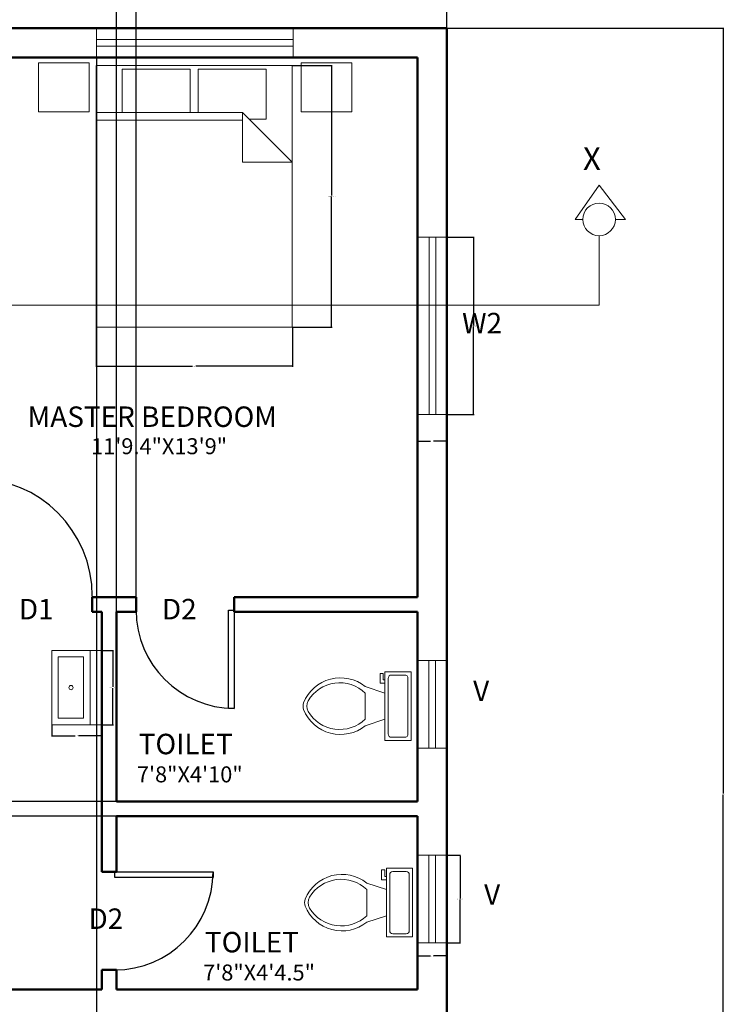
# Model space of a CAD drawing. Units: inches. Extents: x 7359 to 7979, y 33027 to 34263.
# Tile 18 of 32: x 7764 to 7979, y 33329 to 33630. Entities that reach past the tile are written whole.
import ezdxf

# ---------------------------------------------------------------- set-up
doc = ezdxf.new("R2010")
doc.units = ezdxf.units.IN
for name, color, linetype, lineweight in [('A-ANNO-DIMS', 2, 'Continuous', 18), ('A-ANNO-SYMB', 7, 'Continuous', 18), ('A-ANNO-TEXT', 3, 'Continuous', 18), ('A-AREA-IDEN', 7, 'Continuous', 18), ('A-DOOR', 3, 'Continuous', 25), ('A-FLOR-FIXT', 9, 'Continuous', 18), ('A-FURN', 8, 'Continuous', 18), ('A-GLAZ', 4, 'Continuous', 18), ('A-WALL', 7, 'Continuous', 50)]:
    doc.layers.add(name, color=color, linetype=linetype, lineweight=lineweight)
doc.styles.get("Standard").update_dxf_attribs({"font": 'arial.ttf'})
doc.dimstyles.get("Standard").update_dxf_attribs({"dimtxt": 0.18, "dimasz": 0.18, "dimexe": 0.18, "dimexo": 0.0625, "dimgap": 0.09, "dimtad": 0, "dimtih": 1, "dimtoh": 1, "dimdec": 4, "dimzin": 0, "dimdsep": 46, "dimtxsty": 'Standard', "dimcen": 0.09, "dimadec": 0, "dimazin": 0, "dimtfac": 1, "dimtdec": 4, "dimtofl": 0, "dimtmove": 0, "dimatfit": 3, "dimfxl": 1, "dimtolj": 1, "dimtzin": 0, "dimarcsym": 0})

# ---------------------------------------------------------------- blocks, each defined once
blk = doc.blocks.new('*U2')
for p, q in [((0, 0), (0, -100)), ((750, 0), (750, -100))]:
    blk.add_line(p, q)
blk.add_lwpolyline([(0, 0), (0, 750), (43.75, 750), (43.75, 0)], close=True)
blk.add_arc((0, 0), 750, 0, 90)
blk = doc.blocks.new('Bed - Queen')
for p, q in [((0, -80.00003), (0, 0)), ((0, 0), (59.99999, 0)), ((59.99999, 0), (59.99999, -80.00003)), ((7.99999, -1.2), (28.79998, -1.2)), ((7.99999, -14.4), (7.99999, -1.2)), ((28.79998, -1.2), (28.79998, -14.4)), ((31.19999, -1.2), (51.99999, -1.2)), ((31.19999, -14.4), (31.19999, -1.2)), ((51.99999, -1.2), (51.99999, -16.4)), ((0, -14.4), (44.8, -14.4)), ((59.99999, -29.6), (44.8, -14.4)), ((44.8, -14.4), (44.8, -29.6)), ((44.8, -16.8), (0, -16.8)), ((51.99999, -16.4), (46.79936, -16.4)), ((44.8, -29.6), (59.99999, -29.6)), ((59.99999, -80.00003), (0, -80.00003))]:
    blk.add_line(p, q)
blk = doc.blocks.new('Toilet - top')
for p, q in [((9.5, -6), (9.5, -2)), ((-10, -8.5), (-8, -8.5)), ((-10, -9.5), (-10, -8.5)), ((-8, -8.5), (-8, -8)), ((-7, -8), (-7, -9.5)), ((-4, -8), (-6, -14)), ((4, -8), (6, -14)), ((-7, -9.5), (-10, -9.5)), ((4, -14), (-4, -14))]:
    blk.add_line(p, q)
blk.add_lwpolyline([(10.5, -8), (10.5, 0), (-10.5, 0), (-10.5, -8)], close=True)
for points in [[(-9.5, -2), (-9.5, -6)], [(8.5, -1), (-8.5, -1)], [(-8.5, -7), (8.5, -7)]]:
    blk.add_lwpolyline(points)
for centre, radius, start, end in [((-8.62, -1.88), 0.884, 81.8699, 188.1301), ((8.62, -1.88), 0.884, 351.8699, 98.1301), ((-8.62, -6.12), 0.884, 171.8699, 278.1301), ((8.62, -6.12), 0.884, 261.8699, 8.1301), ((3.52, -21.58), 12.17, 141.4691, 247.9714), ((4.2, -21.82), 11.33, 136.3677, 238.9468), ((-3.52, -21.58), 12.17, 292.0284, 38.5307), ((-4.2, -21.82), 11.33, 301.053, 43.6321), ((0, -27.88), 4, 245.7318, 294.2682), ((0, -29), 4, 254.8605, 285.1395)]:
    blk.add_arc(centre, radius, start, end)
blk = doc.blocks.new('TABLE-BEDSIDE')
blk.add_lwpolyline([(0, 15), (15.54, 15), (15.54, 0), (0, 0)], close=True)
blk = doc.blocks.new('BASIN-WALL')
for points in [[(11.75, 22.71), (0, 22.71), (0, 0), (11.75, 0)], [(15.29, 22.71), (11.75, 22.71), (11.75, 0), (15.29, 0)], [(9.75, 20.71), (2, 20.71), (2, 2), (9.75, 2)]]:
    blk.add_lwpolyline(points, close=True)
blk.add_circle((5.88, 11.36), 0.663)
blk = doc.blocks.new('SECTION-HEAD')
for p, q in [((0, 4.98), (7.32, 15.43)), ((7.32, 15.43), (15.39, 4.98)), ((2.34, 4.98), (0, 4.98)), ((12.3, 4.98), (15.39, 4.98))]:
    blk.add_line(p, q)
blk.add_circle((7.32, 4.98), 4.98)
blk = doc.blocks.new('WINDOW-W2-BEDROOM')
for p, q in [((0, 0), (0, 9)), ((60.05, 0), (60.05, 9)), ((60.05, 5.5), (0, 5.5)), ((60.05, 3.5), (0, 3.5))]:
    blk.add_line(p, q)
blk = doc.blocks.new('WINDOW-W2-SIDE')
for p, q in [((0, 54.21), (9, 54.21)), ((3.61, 0), (3.61, 54.21)), ((5.61, 0), (5.61, 54.21)), ((0.22, 0), (9, 0))]:
    blk.add_line(p, q)
blk = doc.blocks.new('VENT-V')
for p, q in [((0, 26.78), (9, 26.78)), ((3.5, 0), (3.5, 26.78)), ((5.5, 0), (5.5, 26.78)), ((0, 0), (9, 0))]:
    blk.add_line(p, q)
blk = doc.blocks.new('*D28')
at = {"layer": 'A-ANNO-DIMS', "color": 0, "lineweight": -2, "transparency": 16777216}
for p, q in [((7846.94, 33615.76), (7859.06, 33615.76)), ((7858.88, 33615.58), (7858.88, 33575.95)), ((7858.88, 33535.94), (7858.88, 33575.57)), ((7846.94, 33535.76), (7859.06, 33535.76))]:
    blk.add_line(p, q, dxfattribs=at)
at = {"layer": 'A-ANNO-DIMS', "color": 0, "transparency": 16777216}
for points in [[(7858.85, 33615.58), (7858.91, 33615.58), (7858.88, 33615.76)], [(7858.85, 33535.94), (7858.91, 33535.94), (7858.88, 33535.76)]]:
    blk.add_solid(points, dxfattribs=at)
at = {"layer": 'Defpoints', "color": 0, "transparency": 16777216}
for p in [(7846.88, 33615.76), (7858.88, 33615.76), (7846.88, 33535.76)]:
    blk.add_point(p, dxfattribs=at)
at = {"layer": 'A-ANNO-DIMS', "color": 0, "transparency": 16777216, "insert": (7858.88, 33575.76), "char_height": 0.18, "attachment_point": 5}
blk.add_mtext('\\A1;QUEEN BED 80 TYP.', dxfattribs=at)
blk = doc.blocks.new('*D29')
at = {"layer": 'A-ANNO-DIMS', "color": 0, "lineweight": -2, "transparency": 16777216}
for p, q in [((7786.88, 33535.7), (7786.88, 33523.58)), ((7846.88, 33535.7), (7846.88, 33523.58)), ((7787.06, 33523.76), (7816.35, 33523.76)), ((7846.7, 33523.76), (7817.4, 33523.76))]:
    blk.add_line(p, q, dxfattribs=at)
at = {"layer": 'A-ANNO-DIMS', "color": 0, "transparency": 16777216}
for points in [[(7787.06, 33523.79), (7787.06, 33523.73), (7786.88, 33523.76)], [(7846.7, 33523.79), (7846.7, 33523.73), (7846.88, 33523.76)]]:
    blk.add_solid(points, dxfattribs=at)
at = {"layer": 'Defpoints', "color": 0, "transparency": 16777216}
for p in [(7786.88, 33535.76), (7846.88, 33535.76), (7846.88, 33523.76)]:
    blk.add_point(p, dxfattribs=at)
at = {"layer": 'A-ANNO-DIMS', "color": 0, "transparency": 16777216, "insert": (7816.88, 33523.76), "char_height": 0.18, "attachment_point": 5}
blk.add_mtext('\\A1;60 TYP.', dxfattribs=at)
blk = doc.blocks.new('*D34')
at = {"layer": 'A-ANNO-DIMS', "color": 0, "lineweight": -2, "transparency": 16777216}
for p, q in [((7894.19, 33374.26), (7898.32, 33374.26)), ((7898.14, 33374.08), (7898.14, 33361.05)), ((7898.14, 33347.66), (7898.14, 33360.69)), ((7894.19, 33347.48), (7898.32, 33347.48))]:
    blk.add_line(p, q, dxfattribs=at)
at = {"layer": 'A-ANNO-DIMS', "color": 0, "transparency": 16777216}
for points in [[(7898.11, 33374.08), (7898.17, 33374.08), (7898.14, 33374.26)], [(7898.11, 33347.66), (7898.17, 33347.66), (7898.14, 33347.48)]]:
    blk.add_solid(points, dxfattribs=at)
at = {"layer": 'Defpoints', "color": 0, "transparency": 16777216}
for p in [(7894.13, 33374.26), (7898.14, 33374.26), (7894.13, 33347.48)]:
    blk.add_point(p, dxfattribs=at)
at = {"layer": 'A-ANNO-DIMS', "color": 0, "transparency": 16777216, "insert": (7898.14, 33360.87), "char_height": 0.18, "attachment_point": 5}
blk.add_mtext('\\A1;VENT V 27 TYP.', dxfattribs=at)
blk = doc.blocks.new('*D35')
at = {"layer": 'A-ANNO-DIMS', "color": 0, "lineweight": -2, "transparency": 16777216}
for p, q in [((7885.13, 33347.42), (7885.13, 33343.28)), ((7894.13, 33347.42), (7894.13, 33343.28)), ((7885.31, 33343.46), (7889.17, 33343.46)), ((7893.95, 33343.46), (7890.08, 33343.46))]:
    blk.add_line(p, q, dxfattribs=at)
at = {"layer": 'A-ANNO-DIMS', "color": 0, "transparency": 16777216}
for points in [[(7885.31, 33343.49), (7885.31, 33343.43), (7885.13, 33343.46)], [(7893.95, 33343.49), (7893.95, 33343.43), (7894.13, 33343.46)]]:
    blk.add_solid(points, dxfattribs=at)
at = {"layer": 'Defpoints', "color": 0, "transparency": 16777216}
for p in [(7885.13, 33347.48), (7894.13, 33347.48), (7894.13, 33343.46)]:
    blk.add_point(p, dxfattribs=at)
at = {"layer": 'A-ANNO-DIMS', "color": 0, "transparency": 16777216, "insert": (7889.63, 33343.46), "char_height": 0.18, "attachment_point": 5}
blk.add_mtext('\\A1;9 TYP.', dxfattribs=at)
blk = doc.blocks.new('*D48')
at = {"layer": 'A-ANNO-DIMS', "color": 0, "lineweight": -2, "transparency": 16777216}
for p, q in [((7788.69, 33436.88), (7792.21, 33436.88)), ((7792.03, 33436.7), (7792.03, 33425.7)), ((7792.03, 33414.34), (7792.03, 33425.34)), ((7788.69, 33414.16), (7792.21, 33414.16))]:
    blk.add_line(p, q, dxfattribs=at)
at = {"layer": 'A-ANNO-DIMS', "color": 0, "transparency": 16777216}
for points in [[(7792, 33436.7), (7792.06, 33436.7), (7792.03, 33436.88)], [(7792, 33414.34), (7792.06, 33414.34), (7792.03, 33414.16)]]:
    blk.add_solid(points, dxfattribs=at)
at = {"layer": 'Defpoints', "color": 0, "transparency": 16777216}
for p in [(7788.63, 33436.88), (7792.03, 33436.88), (7788.63, 33414.16)]:
    blk.add_point(p, dxfattribs=at)
at = {"layer": 'A-ANNO-DIMS', "color": 0, "transparency": 16777216, "insert": (7792.03, 33425.52), "char_height": 0.18, "attachment_point": 5}
blk.add_mtext('\\A1;WALL BASIN 23 TYP.', dxfattribs=at)
blk = doc.blocks.new('*D49')
at = {"layer": 'A-ANNO-DIMS', "color": 0, "lineweight": -2, "transparency": 16777216}
for p, q in [((7773.33, 33414.1), (7773.33, 33410.58)), ((7788.63, 33414.1), (7788.63, 33410.58)), ((7773.51, 33410.76), (7780.46, 33410.76)), ((7788.45, 33410.76), (7781.5, 33410.76))]:
    blk.add_line(p, q, dxfattribs=at)
at = {"layer": 'A-ANNO-DIMS', "color": 0, "transparency": 16777216}
for points in [[(7773.51, 33410.79), (7773.51, 33410.73), (7773.33, 33410.76)], [(7788.45, 33410.79), (7788.45, 33410.73), (7788.63, 33410.76)]]:
    blk.add_solid(points, dxfattribs=at)
at = {"layer": 'Defpoints', "color": 0, "transparency": 16777216}
for p in [(7773.33, 33414.16), (7788.63, 33414.16), (7788.63, 33410.76)]:
    blk.add_point(p, dxfattribs=at)
at = {"layer": 'A-ANNO-DIMS', "color": 0, "transparency": 16777216, "insert": (7780.98, 33410.76), "char_height": 0.18, "attachment_point": 5}
blk.add_mtext('\\A1;15 TYP.', dxfattribs=at)
blk = doc.blocks.new('*D54')
at = {"layer": 'A-ANNO-DIMS', "color": 0, "lineweight": -2, "transparency": 16777216}
for p, q in [((7894.19, 33563.2), (7902.44, 33563.2)), ((7902.26, 33563.02), (7902.26, 33536.27)), ((7902.26, 33509.16), (7902.26, 33535.91)), ((7894.19, 33508.98), (7902.44, 33508.98))]:
    blk.add_line(p, q, dxfattribs=at)
at = {"layer": 'A-ANNO-DIMS', "color": 0, "transparency": 16777216}
for points in [[(7902.23, 33563.02), (7902.29, 33563.02), (7902.26, 33563.2)], [(7902.23, 33509.16), (7902.29, 33509.16), (7902.26, 33508.98)]]:
    blk.add_solid(points, dxfattribs=at)
at = {"layer": 'Defpoints', "color": 0, "transparency": 16777216}
for p in [(7894.13, 33563.2), (7902.26, 33563.2), (7894.13, 33508.98)]:
    blk.add_point(p, dxfattribs=at)
at = {"layer": 'A-ANNO-DIMS', "color": 0, "transparency": 16777216, "insert": (7902.26, 33536.09), "char_height": 0.18, "attachment_point": 5}
blk.add_mtext('\\A1;SIDE W2 54 TYP.', dxfattribs=at)
blk = doc.blocks.new('*D55')
at = {"layer": 'A-ANNO-DIMS', "color": 0, "lineweight": -2, "transparency": 16777216}
for p, q in [((7885.13, 33508.92), (7885.13, 33500.67)), ((7894.13, 33508.92), (7894.13, 33500.67)), ((7885.31, 33500.85), (7889.17, 33500.85)), ((7893.95, 33500.85), (7890.08, 33500.85))]:
    blk.add_line(p, q, dxfattribs=at)
at = {"layer": 'A-ANNO-DIMS', "color": 0, "transparency": 16777216}
for points in [[(7885.31, 33500.88), (7885.31, 33500.82), (7885.13, 33500.85)], [(7893.95, 33500.88), (7893.95, 33500.82), (7894.13, 33500.85)]]:
    blk.add_solid(points, dxfattribs=at)
at = {"layer": 'Defpoints', "color": 0, "transparency": 16777216}
for p in [(7885.13, 33508.98), (7894.13, 33508.98), (7894.13, 33500.85)]:
    blk.add_point(p, dxfattribs=at)
at = {"layer": 'A-ANNO-DIMS', "color": 0, "transparency": 16777216, "insert": (7889.63, 33500.85), "char_height": 0.18, "attachment_point": 5}
blk.add_mtext('\\A1;9 TYP.', dxfattribs=at)
blk = doc.blocks.new('*D66')
at = {"layer": 'A-ANNO-DIMS', "color": 0, "lineweight": -2, "transparency": 16777216}
for p, q in [((7468.73, 33627.22), (7468.73, 33657.24)), ((7468.91, 33657.06), (7681.03, 33657.06)), ((7893.95, 33657.06), (7681.82, 33657.06)), ((7894.13, 33627.22), (7894.13, 33657.24))]:
    blk.add_line(p, q, dxfattribs=at)
at = {"layer": 'A-ANNO-DIMS', "color": 0, "transparency": 16777216}
for points in [[(7468.91, 33657.09), (7468.91, 33657.03), (7468.73, 33657.06)], [(7893.95, 33657.09), (7893.95, 33657.03), (7894.13, 33657.06)]]:
    blk.add_solid(points, dxfattribs=at)
at = {"layer": 'Defpoints', "color": 0, "transparency": 16777216}
for p in [(7894.13, 33657.06), (7468.73, 33627.16), (7894.13, 33627.16)]:
    blk.add_point(p, dxfattribs=at)
at = {"layer": 'A-ANNO-DIMS', "color": 0, "transparency": 16777216, "insert": (7681.43, 33657.06), "char_height": 0.18, "attachment_point": 5}
blk.add_mtext('\\A1;425.4', dxfattribs=at)
blk = doc.blocks.new('*D67')
at = {"layer": 'A-ANNO-DIMS', "color": 0, "lineweight": -2, "transparency": 16777216}
for p, q in [((7894.19, 33627.16), (7978.82, 33627.16)), ((7978.64, 33626.98), (7978.64, 33393.09)), ((7978.64, 33158.84), (7978.64, 33392.73)), ((7894.19, 33158.66), (7978.82, 33158.66))]:
    blk.add_line(p, q, dxfattribs=at)
at = {"layer": 'A-ANNO-DIMS', "color": 0, "transparency": 16777216}
for points in [[(7978.61, 33626.98), (7978.67, 33626.98), (7978.64, 33627.16)], [(7978.61, 33158.84), (7978.67, 33158.84), (7978.64, 33158.66)]]:
    blk.add_solid(points, dxfattribs=at)
at = {"layer": 'Defpoints', "color": 0, "transparency": 16777216}
for p in [(7894.13, 33627.16), (7978.64, 33627.16), (7894.13, 33158.66)]:
    blk.add_point(p, dxfattribs=at)
at = {"layer": 'A-ANNO-DIMS', "color": 0, "transparency": 16777216, "insert": (7978.64, 33392.91), "char_height": 0.18, "attachment_point": 5}
blk.add_mtext('\\A1;468.5', dxfattribs=at)
blk = doc.blocks.new('*D74')
at = {"layer": 'A-ANNO-DIMS', "color": 0, "lineweight": -2, "transparency": 16777216}
for p, q in [((7743.73, 33618.1), (7743.73, 33027.18)), ((7787.03, 33618.1), (7787.03, 33027.18)), ((7743.91, 33027.36), (7765, 33027.36)), ((7786.85, 33027.36), (7765.76, 33027.36))]:
    blk.add_line(p, q, dxfattribs=at)
at = {"layer": 'A-ANNO-DIMS', "color": 0, "transparency": 16777216}
for points in [[(7743.91, 33027.39), (7743.91, 33027.33), (7743.73, 33027.36)], [(7786.85, 33027.39), (7786.85, 33027.33), (7787.03, 33027.36)]]:
    blk.add_solid(points, dxfattribs=at)
at = {"layer": 'Defpoints', "color": 0, "transparency": 16777216}
for p in [(7743.73, 33618.16), (7787.03, 33618.16), (7787.03, 33027.36)]:
    blk.add_point(p, dxfattribs=at)
at = {"layer": 'A-ANNO-DIMS', "color": 0, "transparency": 16777216, "insert": (7765.38, 33027.36), "char_height": 0.18, "attachment_point": 5}
blk.add_mtext('\\A1;43.31', dxfattribs=at)
blk = doc.blocks.new('*D85')
at = {"layer": 'A-ANNO-DIMS', "color": 0, "lineweight": -2, "transparency": 16777216}
for p, q in [((7793.06, 33390.66), (7369.54, 33390.66)), ((7369.72, 33390.48), (7369.72, 33388.59)), ((7793.06, 33386.16), (7369.54, 33386.16)), ((7369.72, 33386.34), (7369.72, 33388.23))]:
    blk.add_line(p, q, dxfattribs=at)
at = {"layer": 'A-ANNO-DIMS', "color": 0, "transparency": 16777216}
for points in [[(7369.69, 33390.48), (7369.75, 33390.48), (7369.72, 33390.66)], [(7369.69, 33386.34), (7369.75, 33386.34), (7369.72, 33386.16)]]:
    blk.add_solid(points, dxfattribs=at)
at = {"layer": 'Defpoints', "color": 0, "transparency": 16777216}
for p in [(7793.13, 33390.66), (7369.72, 33386.16), (7793.13, 33386.16)]:
    blk.add_point(p, dxfattribs=at)
at = {"layer": 'A-ANNO-DIMS', "color": 0, "transparency": 16777216, "insert": (7369.72, 33388.41), "char_height": 0.18, "attachment_point": 5}
blk.add_mtext('\\A1;4.5', dxfattribs=at)
blk = doc.blocks.new('*D88')
at = {"layer": 'A-ANNO-DIMS', "color": 0, "lineweight": -2, "transparency": 16777216}
for p, q in [((7793.126578, 33448.724789), (7793.126578, 33657.242289)), ((7793.306578, 33657.062289), (7795.977151, 33657.062289)), ((7798.946578, 33657.062289), (7796.276005, 33657.062289)), ((7799.126578, 33448.724789), (7799.126578, 33657.242289))]:
    blk.add_line(p, q, dxfattribs=at)
at = {"layer": 'A-ANNO-DIMS', "color": 0, "transparency": 16777216}
for points in [[(7793.306578, 33657.092289), (7793.306578, 33657.032289), (7793.126578, 33657.062289)], [(7798.946578, 33657.092289), (7798.946578, 33657.032289), (7799.126578, 33657.062289)]]:
    blk.add_solid(points, dxfattribs=at)
at = {"layer": 'Defpoints', "color": 0, "transparency": 16777216}
for p in [(7799.126578, 33657.062289), (7793.126578, 33448.662289), (7799.126578, 33448.662289)]:
    blk.add_point(p, dxfattribs=at)
at = {"layer": 'A-ANNO-DIMS', "color": 0, "transparency": 16777216, "insert": (7796.126578, 33657.062289), "char_height": 0.18, "attachment_point": 5}
blk.add_mtext('\\A1;6', dxfattribs=at)

msp = doc.modelspace()

# ---------------------------------------------------------------- linework, layer by layer
at = {"layer": 'A-ANNO-SYMB'}
for p, q in [((7940.6696, 33542.482), (7940.6696, 33563.6906)), ((7406.9423, 33542.482), (7940.6696, 33542.482))]:
    msp.add_line(p, q, dxfattribs=at)
at = {"layer": 'A-WALL'}
for p, q in [((7468.7266, 33627.1623), (7894.1266, 33627.1623)), ((7894.1266, 33627.1623), (7894.1266, 33158.6623)), ((7743.7266, 33618.1623), (7885.1266, 33618.1623)), ((7885.1266, 33618.1623), (7885.1266, 33453.1623)), ((7785.7266, 33453.1623), (7799.1266, 33453.1623)), ((7785.7266, 33453.1623), (7785.7266, 33448.6623)), ((7799.1266, 33448.6623), (7799.1266, 33453.1623)), ((7829.1266, 33453.1623), (7885.1266, 33453.1623)), ((7829.1266, 33448.6623), (7829.1266, 33453.1623)), ((7785.7266, 33448.6623), (7788.6266, 33448.6623)), ((7788.6266, 33448.6623), (7788.6266, 33369.1623)), ((7793.1266, 33448.6623), (7799.1266, 33448.6623)), ((7793.1266, 33448.6623), (7793.1266, 33390.6623)), ((7829.1266, 33448.6623), (7885.1266, 33448.6623)), ((7885.1266, 33448.6623), (7885.1266, 33390.6623)), ((7793.1266, 33390.6623), (7885.1266, 33390.6623)), ((7793.1266, 33386.1623), (7885.1266, 33386.1623)), ((7793.1266, 33386.1623), (7793.1266, 33369.1623)), ((7885.1266, 33386.1623), (7885.1266, 33333.1623)), ((7788.6266, 33369.1623), (7793.1266, 33369.1623)), ((7788.6266, 33339.1623), (7788.6266, 33333.1623)), ((7788.6266, 33339.1623), (7793.1266, 33339.1623)), ((7793.1266, 33339.1623), (7793.1266, 33333.1623)), ((7699.6266, 33333.1623), (7788.6266, 33333.1623)), ((7793.1266, 33333.1623), (7885.1266, 33333.1623))]:
    msp.add_line(p, q, dxfattribs=at)

# ---------------------------------------------------------------- block references
at = {"layer": 'A-ANNO-SYMB'}
msp.add_blockref('SECTION-HEAD', (7933.3494, 33563.6904), dxfattribs=at)
at = {"layer": 'A-DOOR', "xscale": 0.0479999999999996, "yscale": 0.0479999999999996, "zscale": 0.0479999999999996}
msp.add_blockref('*U2', (7749.7266, 33453.4623), dxfattribs=at)
at = {"layer": 'A-DOOR', "xscale": 0.0399999999999999, "yscale": 0.0399999999999999, "zscale": 0.0399999999999999}
for p, rotation in [((7829.1266, 33449.1623), 180), ((7792.6266, 33369.1623), 270)]:
    msp.add_blockref('*U2', p, dxfattribs=dict(at, rotation=rotation))
at = {"layer": 'A-FLOR-FIXT'}
msp.add_blockref('BASIN-WALL', (7773.3331, 33414.1634), dxfattribs=at)
at = {"layer": 'A-FLOR-FIXT', "rotation": 270}
for p in [(7883.1963, 33419.8305), (7883.6459, 33359.754)]:
    msp.add_blockref('Toilet - top', p, dxfattribs=at)
at = {"layer": 'A-FURN'}
for name, p in [('TABLE-BEDSIDE', (7769.2358, 33601.5164)), ('Bed - Queen', (7786.8755, 33615.7623)), ('TABLE-BEDSIDE', (7849.576, 33601.5164))]:
    msp.add_blockref(name, p, dxfattribs=at)
at = {"layer": 'A-GLAZ'}
for name, p in [('WINDOW-W2-BEDROOM', (7787.0341, 33618.1624)), ('WINDOW-W2-SIDE', (7885.1261, 33508.9844)), ('VENT-V', (7885.1261, 33406.9614)), ('VENT-V', (7885.1261, 33347.4774))]:
    msp.add_blockref(name, p, dxfattribs=at)

# ---------------------------------------------------------------- texts
at = {"layer": 'A-ANNO-SYMB'}
msp.add_text('X', height=6.9459, dxfattribs=at).set_placement((7935.7493, 33583.7843))
at = {"layer": 'A-ANNO-TEXT'}
for s, height, p in [('W2', 6.25941, (7898.7689, 33533.8335)), ('D1', 6.25941, (7763.2844, 33446.3685)), ('D2', 6.25941, (7807.0172, 33446.3685)), ('V', 6.2594, (7902.1499, 33421.3714)), ('V', 6.2594, (7905.5059, 33359.0973)), ('D2', 6.25941, (7784.5645, 33351.706))]:
    msp.add_text(s, height=height, dxfattribs=at).set_placement(p)
at = {"layer": 'A-AREA-IDEN'}
for s, height, p in [('MASTER BEDROOM', 6.259411, (7765.9469, 33505.2058)), ('11\'9.4"X13\'9"', 4.885549, (7785.3446, 33496.8715)), ('TOILET', 6.25941, (7799.9158, 33405.1242)), ('7\'8"X4\'10"', 4.88555, (7799.3526, 33396.5298)), ('TOILET', 6.25941, (7820.167, 33344.5373)), ('7\'8"X4\'4.5"', 4.885549, (7819.6038, 33335.9429))]:
    msp.add_text(s, height=height, dxfattribs=at).set_placement(p)

# ---------------------------------------------------------------- dimensions: what is measured, and where the dimension line sits
at = {"layer": 'A-ANNO-DIMS'}
for base, p1, p2, override, picture, middle in [((7894.1266, 33657.0623), (7468.7266, 33627.1623), (7894.1266, 33627.1623), {"dimdec": 1, "dimlfac": 1, "dimrnd": 0, "dimzin": 0, "dimdsep": 46, "dimlunit": 2}, '*D66', (7681.4266, 33657.0623)), ((7799.1266, 33657.0623), (7793.1266, 33448.6623), (7799.1266, 33448.6623), {"dimdec": 0, "dimlfac": 1, "dimrnd": 0, "dimzin": 0, "dimdsep": 46, "dimlunit": 2}, '*D88', (7796.1266, 33657.0623)), ((7787.0342, 33027.3568), (7743.7266, 33618.1623), (7787.0342, 33618.1623), {"dimdec": 2, "dimlfac": 1, "dimrnd": 0, "dimzin": 0, "dimdsep": 46, "dimlunit": 2}, '*D74', (7765.3804, 33027.3568))]:
    dim = msp.add_linear_dim(base=base, p1=p1, p2=p2, dimstyle='Standard', override=override, dxfattribs=at)
    dim.commit()
    dim.dimension.update_dxf_attribs({"geometry": picture, "text_midpoint": middle})
for base, p1, p2, picture, middle in [((7978.6371, 33627.1623), (7894.1266, 33158.6623), (7894.1266, 33627.1623), '*D67', (7978.6371, 33392.9123)), ((7369.7217, 33386.1623), (7793.1266, 33390.6623), (7793.1266, 33386.1623), '*D85', (7369.7217, 33388.4123))]:
    dim = msp.add_linear_dim(base=base, p1=p1, p2=p2, angle=90, dimstyle='Standard', override={"dimdec": 1, "dimlfac": 1, "dimrnd": 0, "dimzin": 0, "dimdsep": 46, "dimlunit": 2}, dxfattribs=at)
    dim.commit()
    dim.dimension.update_dxf_attribs({"geometry": picture, "text_midpoint": middle})
for base, p1, p2, text, picture, middle in [((7858.8755, 33615.7623), (7846.8755, 33535.7623), (7846.8755, 33615.7623), 'QUEEN BED <> TYP.', '*D28', (7858.8755, 33575.7623)), ((7902.2585, 33563.1972), (7894.1266, 33508.9845), (7894.1266, 33563.1972), 'SIDE W2 <> TYP.', '*D54', (7902.2585, 33536.0909)), ((7792.0337, 33436.877), (7788.6266, 33414.1632), (7788.6266, 33436.877), 'WALL BASIN <> TYP.', '*D48', (7792.0337, 33425.5201)), ((7898.1434, 33374.2563), (7894.1266, 33347.4775), (7894.1266, 33374.2563), 'VENT V <> TYP.', '*D34', (7898.1434, 33360.8669))]:
    dim = msp.add_linear_dim(base=base, p1=p1, p2=p2, angle=90, text=text, dimstyle='Standard', override={"dimdec": 0, "dimlfac": 1, "dimrnd": 0, "dimzin": 0, "dimdsep": 46, "dimlunit": 2}, dxfattribs=at)
    dim.commit()
    dim.dimension.update_dxf_attribs({"geometry": picture, "text_midpoint": middle})
for base, p1, p2, picture, middle in [((7846.8755, 33523.7623), (7786.8755, 33535.7623), (7846.8755, 33535.7623), '*D29', (7816.8755, 33523.7623)), ((7894.1266, 33500.8526), (7885.1266, 33508.9845), (7894.1266, 33508.9845), '*D55', (7889.6266, 33500.8526)), ((7788.6266, 33410.7561), (7773.3328, 33414.1632), (7788.6266, 33414.1632), '*D49', (7780.9797, 33410.7561)), ((7894.1266, 33343.4607), (7885.1266, 33347.4775), (7894.1266, 33347.4775), '*D35', (7889.6266, 33343.4607))]:
    dim = msp.add_linear_dim(base=base, p1=p1, p2=p2, text='<> TYP.', dimstyle='Standard', override={"dimdec": 0, "dimlfac": 1, "dimrnd": 0, "dimzin": 0, "dimdsep": 46, "dimlunit": 2}, dxfattribs=at)
    dim.commit()
    dim.dimension.update_dxf_attribs({"geometry": picture, "text_midpoint": middle})

doc.saveas('drawing.dxf')
